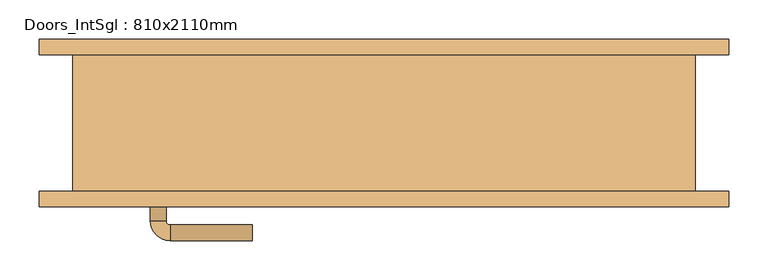
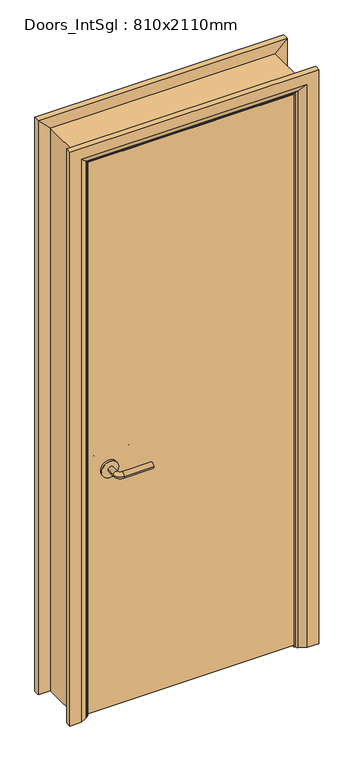
"""IFC4 building model written with IfcOpenShell, lengths in millimetres: door geometry, Doors_IntSgl : 810x2110mm."""

from ifc_helpers import new_model, si_unit, point, frame, frame_2d, origin, place, context, project, spatial, polyline, circle_curve, ellipse_curve, trimmed, segment, composite_curve, outline, extrude, faceted_brep, source, transform, mapped, element, save
from ifc_brep_helpers import plane_surface, cylinder_surface, revolved_surface, advanced_brep


def doors_intsgl_810x2110mm_f0bad3dc(model_context):
    return source(origin(), model_context, "Body", "SolidModel", [
        advanced_brep(
        [(-298.0, -40.868, 900.0), (-278.0, -40.868, 900.0), (-298.0, -10.868, 900.0), (-278.0, -10.868, 900.0), (-273.0, -5.868, 900.0), (-273.0, 14.132, 900.0), (-168.0, 14.132, 900.0), (-168.0, -5.868, 900.0)],
        [
            (0, 1, circle_curve(frame((-288.0, -40.868, 900.0), z_axis=(0.0, -1.0, 0.0), x_axis=(1.0, 0.0, 0.0)), 10.0)),
            (1, 0, circle_curve(frame((-288.0, -40.868, 900.0), z_axis=(0.0, -1.0, 0.0), x_axis=(1.0, 0.0, 0.0)), 10.0)),
            (0, 2),
            (2, 3, circle_curve(frame((-288.0, -10.868, 900.0), z_axis=(0.0, -1.0, 0.0), x_axis=(1.0, 0.0, 0.0)), 10.0)),
            (3, 1),
            (3, 2, circle_curve(frame((-288.0, -10.868, 900.0), z_axis=(0.0, -1.0, 0.0), x_axis=(1.0, 0.0, 0.0)), 10.0)),
            (4, 3, circle_curve(frame((-273.0, -10.868, 900.0), z_axis=(0.0, 0.0, 1.0), x_axis=(-1.0, 0.0, 0.0)), 5.0)),
            (2, 5, circle_curve(frame((-273.0, -10.868, 900.0), z_axis=(0.0, 0.0, -1.0), x_axis=(-1.0, 0.0, 0.0)), 25.0)),
            (5, 4, circle_curve(frame((-273.0, 4.132, 900.0), z_axis=(-1.0, 0.0, 0.0), x_axis=(0.0, -1.0, 0.0)), 10.0)),
            (4, 5, circle_curve(frame((-273.0, 4.132, 900.0), z_axis=(-1.0, 0.0, 0.0), x_axis=(0.0, -1.0, 0.0)), 10.0)),
            (6, 7, circle_curve(frame((-168.0, 4.132, 900.0), z_axis=(1.0, 0.0, 0.0), x_axis=(0.0, -1.0, 0.0)), 10.0)),
            (7, 6, circle_curve(frame((-168.0, 4.132, 900.0), z_axis=(1.0, 0.0, 0.0), x_axis=(0.0, -1.0, 0.0)), 10.0)),
            (5, 6),
            (7, 4),
        ],
        [
            plane_surface(frame((-288.0, -40.868, 900.0), z_axis=(0.0, -1.0, 0.0), x_axis=(0.0, 0.0, 1.0))),
            cylinder_surface(frame((-288.0, -40.868, 900.0), z_axis=(0.0, -1.0, 0.0), x_axis=(1.0, 0.0, 0.0)), 10.0),
            revolved_surface(trimmed(ellipse_curve(frame((-288.0, -10.868, 900.0), z_axis=(0.0, -1.0, 0.0), x_axis=(1.0, 0.0, 0.0)), 10.0, 10.0), [point((-298.0, -10.868, 900.0))], [point((-278.0, -10.868, 900.0))], True, "CARTESIAN"), (-273.0, -10.868, 900.0), (0.0, 0.0, -1.0)),
            revolved_surface(trimmed(ellipse_curve(frame((-288.0, -10.868, 900.0), z_axis=(0.0, -1.0, 0.0), x_axis=(1.0, 0.0, 0.0)), 10.0, 10.0), [point((-278.0, -10.868, 900.0))], [point((-298.0, -10.868, 900.0))], True, "CARTESIAN"), (-273.0, -10.868, 900.0), (0.0, 0.0, -1.0)),
            plane_surface(frame((-168.0, 4.132, 900.0), z_axis=(1.0, 0.0, 0.0), x_axis=(0.0, 0.0, 1.0))),
            cylinder_surface(frame((-273.0, 4.132, 900.0), z_axis=(-1.0, 0.0, 0.0), x_axis=(0.0, -1.0, 0.0)), 10.0),
        ],
        [
            (0, [[1, 2]]),
            (1, [[-1, 3, 4, 5]]),
            (1, [[-2, -5, 6, -3]]),
            (2, [[7, -4, 8, 9]]),
            (3, [[-8, -6, -7, 10]]),
            (4, [[11, 12]]),
            (5, [[-9, 13, -12, 14]]),
            (5, [[-10, -14, -11, -13]]),
        ],
    ),
        extrude(outline(composite_curve([segment(trimmed(circle_curve(frame_2d((900.0, -290.5)), 30.0), [point((900.0, -320.5))], [point((900.0, -260.5))], False, "CARTESIAN"), True, "CONTINUOUS"), segment(trimmed(circle_curve(frame_2d((900.0, -290.5)), 30.0), [point((900.0, -260.5))], [point((900.0, -320.5))], False, "CARTESIAN"), True, "CONTINUOUS")], self_intersect=False)), frame((0.0, -48.868, 0.0), z_axis=(0.0, 1.0, 0.0), x_axis=(0.0, 0.0, 1.0)), (0.0, 0.0, 1.0), 8.0),
        advanced_brep(
        [(-298.0, -94.868, 900.0), (-278.0, -94.868, 900.0), (-278.0, -124.868, 900.0), (-298.0, -124.868, 900.0), (-273.0, -129.868, 900.0), (-273.0, -149.868, 900.0), (-168.0, -149.868, 900.0), (-168.0, -129.868, 900.0)],
        [
            (0, 1, circle_curve(frame((-288.0, -94.868, 900.0), z_axis=(0.0, 1.0, 0.0), x_axis=(1.0, 0.0, 0.0)), 10.0)),
            (1, 0, circle_curve(frame((-288.0, -94.868, 900.0), z_axis=(0.0, 1.0, 0.0), x_axis=(1.0, 0.0, 0.0)), 10.0)),
            (1, 2),
            (2, 3, circle_curve(frame((-288.0, -124.868, 900.0), z_axis=(0.0, 1.0, 0.0), x_axis=(1.0, 0.0, 0.0)), 10.0)),
            (3, 0),
            (3, 2, circle_curve(frame((-288.0, -124.868, 900.0), z_axis=(0.0, 1.0, 0.0), x_axis=(1.0, 0.0, 0.0)), 10.0)),
            (4, 5, circle_curve(frame((-273.0, -139.868, 900.0), z_axis=(-1.0, 0.0, 0.0), x_axis=(0.0, 1.0, 0.0)), 10.0)),
            (5, 3, circle_curve(frame((-273.0, -124.868, 900.0), z_axis=(0.0, 0.0, -1.0), x_axis=(-1.0, 0.0, 0.0)), 25.0)),
            (2, 4, circle_curve(frame((-273.0, -124.868, 900.0), z_axis=(0.0, 0.0, 1.0), x_axis=(-1.0, 0.0, 0.0)), 5.0)),
            (5, 4, circle_curve(frame((-273.0, -139.868, 900.0), z_axis=(-1.0, 0.0, 0.0), x_axis=(0.0, 1.0, 0.0)), 10.0)),
            (6, 7, circle_curve(frame((-168.0, -139.868, 900.0), z_axis=(1.0, 0.0, 0.0), x_axis=(0.0, 1.0, 0.0)), 10.0)),
            (7, 6, circle_curve(frame((-168.0, -139.868, 900.0), z_axis=(1.0, 0.0, 0.0), x_axis=(0.0, 1.0, 0.0)), 10.0)),
            (4, 7),
            (6, 5),
        ],
        [
            plane_surface(frame((-288.0, -94.868, 900.0), z_axis=(0.0, 1.0, 0.0), x_axis=(0.0, 0.0, 1.0))),
            cylinder_surface(frame((-288.0, -94.868, 900.0), z_axis=(0.0, 1.0, 0.0), x_axis=(1.0, 0.0, 0.0)), 10.0),
            revolved_surface(trimmed(ellipse_curve(frame((-288.0, -124.868, 900.0), z_axis=(0.0, -1.0, 0.0), x_axis=(1.0, 0.0, 0.0)), 10.0, 10.0), [point((-298.0, -124.868, 900.0))], [point((-278.0, -124.868, 900.0))], True, "CARTESIAN"), (-273.0, -124.868, 900.0), (0.0, 0.0, -1.0)),
            revolved_surface(trimmed(ellipse_curve(frame((-288.0, -124.868, 900.0), z_axis=(0.0, -1.0, 0.0), x_axis=(1.0, 0.0, 0.0)), 10.0, 10.0), [point((-278.0, -124.868, 900.0))], [point((-298.0, -124.868, 900.0))], True, "CARTESIAN"), (-273.0, -124.868, 900.0), (0.0, 0.0, -1.0)),
            plane_surface(frame((-168.0, -139.868, 900.0), z_axis=(1.0, 0.0, 0.0), x_axis=(0.0, 0.0, 1.0))),
            cylinder_surface(frame((-273.0, -139.868, 900.0), z_axis=(-1.0, 0.0, 0.0), x_axis=(0.0, 1.0, 0.0)), 10.0),
        ],
        [
            (0, [[1, 2]]),
            (1, [[3, 4, 5, -2]]),
            (1, [[-5, 6, -3, -1]]),
            (2, [[7, 8, -4, 9]]),
            (3, [[10, -9, -6, -8]]),
            (4, [[11, 12]]),
            (5, [[13, -11, 14, -7]]),
            (5, [[-14, -12, -13, -10]]),
        ],
    ),
        extrude(outline(composite_curve([segment(trimmed(circle_curve(frame_2d((900.0, -290.5)), 30.0), [point((900.0, -320.5))], [point((900.0, -260.5))], False, "CARTESIAN"), True, "CONTINUOUS"), segment(trimmed(circle_curve(frame_2d((900.0, -290.5)), 30.0), [point((900.0, -260.5))], [point((900.0, -320.5))], False, "CARTESIAN"), True, "CONTINUOUS")], self_intersect=False)), frame((0.0, -94.868, 0.0), z_axis=(0.0, 1.0, 0.0), x_axis=(0.0, 0.0, 1.0)), (0.0, 0.0, 1.0), 8.0),
        extrude(outline(polyline([(363.0, -48.868), (363.0, -86.868), (-363.0, -86.868), (-363.0, -48.868), (363.0, -48.868)])), frame((0.0, 0.0, 8.0), z_axis=(0.0, 0.0, 1.0), x_axis=(1.0, 0.0, 0.0)), (0.0, 0.0, 1.0), 2060.0),
        advanced_brep(
        [(440.0, -106.868, 0.0), (400.0, -106.868, 0.0), (374.0, -92.868, 0.0), (370.0, -86.868, 0.0), (440.0, -86.868, 0.0), (440.0, -86.868, 2145.0), (440.0, -106.868, 2145.0), (370.0, -86.868, 2075.0), (-370.0, -86.868, 2075.0), (-370.0, -86.868, 0.0), (-440.0, -86.868, 0.0), (-440.0, -86.868, 2145.0), (374.0, -92.868, 2079.0), (400.0, -106.868, 2105.0), (-440.0, -106.868, 2145.0), (-440.0, -106.868, 0.0), (-400.0, -106.868, 0.0), (-400.0, -106.868, 2105.0), (-374.0, -92.868, 2079.0), (-374.0, -92.868, 0.0)],
        [
            (0, 1),
            (1, 2),
            (2, 3, circle_curve(frame((378.0, -85.868, 0.0), z_axis=(0.0, 0.0, -1.0), x_axis=(1.0, 0.0, 0.0)), 8.0622577)),
            (3, 4),
            (4, 0),
            (4, 5),
            (5, 6),
            (6, 0),
            (3, 7),
            (7, 8),
            (8, 9),
            (9, 10),
            (10, 11),
            (11, 5),
            (2, 12),
            (12, 7, ellipse_curve(frame((378.0, -85.868, 2083.0), z_axis=(0.7071067811865475, 0.0, -0.7071067811865475), x_axis=(-0.7071067811865474, 0.0, -0.7071067811865476)), 11.4017543, 8.0622577)),
            (1, 13),
            (13, 12),
            (6, 14),
            (14, 15),
            (15, 16),
            (16, 17),
            (17, 13),
            (11, 14),
            (12, 18),
            (18, 8, ellipse_curve(frame((-378.0, -85.868, 2083.0), z_axis=(0.7071067811865475, 0.0, 0.7071067811865475), x_axis=(0.7071067811865476, 0.0, -0.7071067811865474)), 11.4017543, 8.0622577)),
            (17, 18),
            (15, 10),
            (9, 19, circle_curve(frame((-378.0, -85.868, 0.0), z_axis=(0.0, 0.0, -1.0), x_axis=(-1.0, 0.0, 0.0)), 8.0622577)),
            (19, 16),
            (18, 19),
        ],
        [
            plane_surface(frame((370.0, -86.868, 0.0), z_axis=(0.0, 0.0, -1.0), x_axis=(0.0, 1.0, 0.0))),
            plane_surface(frame((440.0, -106.868, 0.0), z_axis=(1.0, 0.0, 0.0), x_axis=(0.0, 0.0, 1.0))),
            plane_surface(frame((440.0, -86.868, 0.0), z_axis=(0.0, 1.0, 0.0), x_axis=(0.0, 0.0, 1.0))),
            cylinder_surface(frame((378.0, -85.868, 0.0), z_axis=(0.0, 0.0, -1.0), x_axis=(1.0, 0.0, 0.0)), 8.0622577),
            plane_surface(frame((374.0, -92.868, 0.0), z_axis=(-0.4740998230350126, -0.880471099922178, 0.0), x_axis=(0.0, 0.0, 1.0))),
            plane_surface(frame((400.0, -106.868, 0.0), z_axis=(0.0, -1.0, 0.0), x_axis=(0.0, 0.0, 1.0))),
            plane_surface(frame((440.0, -106.868, 2145.0), z_axis=(0.0, 0.0, 1.0), x_axis=(-1.0, 0.0, 0.0))),
            cylinder_surface(frame((370.0, -85.868, 2083.0), z_axis=(1.0, 0.0, 0.0), x_axis=(0.0, 0.0, 1.0)), 8.0622577),
            plane_surface(frame((374.0, -92.868, 2079.0), z_axis=(0.0, -0.8804710999221764, -0.4740998230350154), x_axis=(-1.0, 0.0, 0.0))),
            plane_surface(frame((-370.0, -86.868, 0.0), z_axis=(0.0, 0.0, -1.0), x_axis=(0.0, 1.0, 0.0))),
            plane_surface(frame((-440.0, -106.868, 2145.0), z_axis=(-1.0, 0.0, 0.0), x_axis=(0.0, 0.0, -1.0))),
            cylinder_surface(frame((-378.0, -85.868, 2075.0), z_axis=(0.0, 0.0, 1.0), x_axis=(-1.0, 0.0, 0.0)), 8.0622577),
            plane_surface(frame((-374.0, -92.868, 2079.0), z_axis=(0.47409982303501824, -0.8804710999221749, 0.0), x_axis=(0.0, 0.0, -1.0))),
        ],
        [
            (0, [[1, 2, 3, 4, 5]]),
            (1, [[6, 7, 8, -5]]),
            (2, [[9, 10, 11, 12, 13, 14, -6, -4]]),
            (3, [[15, 16, -9, -3]]),
            (4, [[17, 18, -15, -2]]),
            (5, [[-8, 19, 20, 21, 22, 23, -17, -1]]),
            (6, [[-14, 24, -19, -7]]),
            (7, [[25, 26, -10, -16]]),
            (8, [[-23, 27, -25, -18]]),
            (9, [[28, -12, 29, 30, -21]]),
            (10, [[-13, -28, -20, -24]]),
            (11, [[31, -29, -11, -26]]),
            (12, [[-22, -30, -31, -27]]),
        ],
    ),
        extrude(outline(polyline([(0.0, -346.0), (2051.0, -346.0), (2051.0, 346.0), (0.0, 346.0), (0.0, 365.0), (2070.0, 365.0), (2070.0, -365.0), (0.0, -365.0), (0.0, -346.0)])), frame((0.0, -46.868, 0.0), z_axis=(0.0, 1.0, 0.0), x_axis=(0.0, 0.0, 1.0)), (0.0, 0.0, 1.0), 32.0),
        advanced_brep(
        [(-440.0, 106.868, 0.0), (-400.0, 106.868, 0.0), (-374.0, 92.868, 0.0), (-370.0, 86.868, 0.0), (-440.0, 86.868, 0.0), (-440.0, 86.868, 2145.0), (-440.0, 106.868, 2145.0), (-370.0, 86.868, 2075.0), (-374.0, 92.868, 2079.0), (-400.0, 106.868, 2105.0), (440.0, 86.868, 2145.0), (440.0, 106.868, 2145.0), (370.0, 86.868, 2075.0), (374.0, 92.868, 2079.0), (400.0, 106.868, 2105.0), (440.0, 106.868, 0.0), (440.0, 86.868, 0.0), (370.0, 86.868, 0.0), (374.0, 92.868, 0.0), (400.0, 106.868, 0.0)],
        [
            (0, 1),
            (1, 2),
            (2, 3, circle_curve(frame((-378.0, 85.868, 0.0), z_axis=(0.0, 0.0, -1.0), x_axis=(-1.0, 0.0, 0.0)), 8.0622577)),
            (3, 4),
            (4, 0),
            (4, 5),
            (5, 6),
            (6, 0),
            (3, 7),
            (7, 5),
            (2, 8),
            (8, 7, ellipse_curve(frame((-378.0, 85.868, 2083.0), z_axis=(-0.7071067811865475, 0.0, -0.7071067811865475), x_axis=(0.7071067811865474, 0.0, -0.7071067811865476)), 11.4017543, 8.0622577)),
            (1, 9),
            (9, 8),
            (6, 9),
            (5, 10),
            (10, 11),
            (11, 6),
            (7, 12),
            (12, 10),
            (8, 13),
            (13, 12, ellipse_curve(frame((378.0, 85.868, 2083.0), z_axis=(-0.7071067811865475, 0.0, 0.7071067811865475), x_axis=(-0.7071067811865476, 0.0, -0.7071067811865474)), 11.4017543, 8.0622577)),
            (9, 14),
            (14, 13),
            (11, 14),
            (15, 16),
            (16, 17),
            (17, 18, circle_curve(frame((378.0, 85.868, 0.0), z_axis=(0.0, 0.0, -1.0), x_axis=(1.0, 0.0, 0.0)), 8.0622577)),
            (18, 19),
            (19, 15),
            (10, 16),
            (15, 11),
            (12, 17),
            (13, 18),
            (14, 19),
        ],
        [
            plane_surface(frame((-370.0, 159.6690989, 0.0), z_axis=(0.0, 0.0, -1.0), x_axis=(1.0, 0.0, 0.0))),
            plane_surface(frame((-440.0, 106.868, 0.0), z_axis=(-1.0, 0.0, 0.0), x_axis=(0.0, 0.0, 1.0))),
            plane_surface(frame((-440.0, 86.868, 0.0), z_axis=(0.0, -1.0, 0.0), x_axis=(0.0, 0.0, 1.0))),
            cylinder_surface(frame((-378.0, 85.868, 0.0), z_axis=(0.0, 0.0, -1.0), x_axis=(-1.0, 0.0, 0.0)), 8.0622577),
            plane_surface(frame((-374.0, 92.868, 0.0), z_axis=(0.4740998230350183, 0.8804710999221749, 0.0), x_axis=(0.0, 0.0, 1.0))),
            plane_surface(frame((-400.0, 106.868, 0.0), z_axis=(0.0, 1.0, 0.0), x_axis=(0.0, 0.0, 1.0))),
            plane_surface(frame((-440.0, 106.868, 2145.0), z_axis=(0.0, 0.0, 1.0), x_axis=(1.0, 0.0, 0.0))),
            plane_surface(frame((-440.0, 86.868, 2145.0), z_axis=(0.0, -1.0, 0.0), x_axis=(1.0, 0.0, 0.0))),
            cylinder_surface(frame((-370.0, 85.868, 2083.0), z_axis=(-1.0, 0.0, 0.0), x_axis=(0.0, 0.0, 1.0)), 8.0622577),
            plane_surface(frame((-374.0, 92.868, 2079.0), z_axis=(0.0, 0.8804710999221749, -0.4740998230350183), x_axis=(1.0, 0.0, 0.0))),
            plane_surface(frame((-400.0, 106.868, 2105.0), z_axis=(0.0, 1.0, 0.0), x_axis=(1.0, 0.0, 0.0))),
            plane_surface(frame((370.0, 159.6690989, 0.0), z_axis=(0.0, 0.0, -1.0), x_axis=(-1.0, 0.0, 0.0))),
            plane_surface(frame((440.0, 106.868, 2145.0), z_axis=(1.0, 0.0, 0.0), x_axis=(0.0, 0.0, -1.0))),
            plane_surface(frame((440.0, 86.868, 2145.0), z_axis=(0.0, -1.0, 0.0), x_axis=(0.0, 0.0, -1.0))),
            cylinder_surface(frame((378.0, 85.868, 2075.0), z_axis=(0.0, 0.0, 1.0), x_axis=(1.0, 0.0, 0.0)), 8.0622577),
            plane_surface(frame((374.0, 92.868, 2079.0), z_axis=(-0.4740998230350183, 0.8804710999221749, 0.0), x_axis=(0.0, 0.0, -1.0))),
            plane_surface(frame((400.0, 106.868, 2105.0), z_axis=(0.0, 1.0, 0.0), x_axis=(0.0, 0.0, -1.0))),
        ],
        [
            (0, [[1, 2, 3, 4, 5]]),
            (1, [[6, 7, 8, -5]]),
            (2, [[9, 10, -6, -4]]),
            (3, [[11, 12, -9, -3]]),
            (4, [[13, 14, -11, -2]]),
            (5, [[-8, 15, -13, -1]]),
            (6, [[16, 17, 18, -7]]),
            (7, [[19, 20, -16, -10]]),
            (8, [[21, 22, -19, -12]]),
            (9, [[23, 24, -21, -14]]),
            (10, [[-18, 25, -23, -15]]),
            (11, [[26, 27, 28, 29, 30]]),
            (12, [[31, -26, 32, -17]]),
            (13, [[33, -27, -31, -20]]),
            (14, [[34, -28, -33, -22]]),
            (15, [[35, -29, -34, -24]]),
            (16, [[-32, -30, -35, -25]]),
        ],
    ),
        faceted_brep([(-365.0, -86.868, 0.0), (-397.0, -86.868, 0.0), (-397.0, 86.868, 0.0), (-365.0, 86.868, 0.0), (-365.0, 86.868, 2070.0), (-365.0, -86.868, 2070.0), (-397.0, 86.868, 2102.0), (-397.0, -86.868, 2102.0), (365.0, 86.868, 2070.0), (365.0, -86.868, 2070.0), (397.0, 86.868, 2102.0), (397.0, -86.868, 2102.0), (365.0, -86.868, 0.0), (365.0, 86.868, 0.0), (397.0, 86.868, 0.0), (397.0, -86.868, 0.0)], [[[0, 1, 2, 3]], [[3, 4, 5, 0]], [[2, 6, 4, 3]], [[1, 7, 6, 2]], [[0, 5, 7, 1]], [[4, 8, 9, 5]], [[6, 10, 8, 4]], [[7, 11, 10, 6]], [[5, 9, 11, 7]], [[12, 13, 14, 15]], [[8, 13, 12, 9]], [[10, 14, 13, 8]], [[11, 15, 14, 10]], [[9, 12, 15, 11]]]),
    ])


if __name__ == "__main__":
    model = new_model("IFC4")
    model_context = context("Model", 3, world=origin())
    ifc_project = project(units=[si_unit("LENGTHUNIT", "METRE", prefix="MILLI")], contexts=[model_context])
    site = spatial("IfcSite", under=ifc_project)
    building = spatial("IfcBuilding", under=site)
    placement = place(None, origin())
    doors_intsgl_810x2110mm_shape = doors_intsgl_810x2110mm_f0bad3dc(model_context)
    element("IfcDoor", 1, ObjectType="Doors_IntSgl : 810x2110mm", at=placement, inside=building, context=model_context, shape_type="MappedRepresentation", body=[
        mapped(doors_intsgl_810x2110mm_shape, transform((0.0, 0.0, 0.0), x_axis=(1.0, 0.0, 0.0), y_axis=(0.0, 1.0, 0.0), z_axis=(0.0, 0.0, 1.0))),
    ])
    save(model, "model.ifc")

# Revit data of these elements
# Type "Doors_IntSgl : 810x2110mm"
#   Construction Type Id = "MDOOR"
#   Type Mark = "42"
#   Type Comments = "Internal Single"
#   Operation = "SingleSwingRight"
#   Manufacturer = "Revit"
#   Keynote = "L20"
#   Description = "Internal Single Door"
#   Analytic Construction = "Metal"
#   UnderCut = 0.026247 ft
#   Tolerance = 0.006562 ft
#   Thickness = 0.124672 ft
#   Thermal Resistance (R) = 0.270117 (m²·K)/W
#   Structural Tolerance = 0.026247 ft
#   StopDepth = 0.104987 ft
#   Stop Thickness = 0.062336 ft
#   Rough Width = 2.65748 ft
#   Rough Height = 6.922572 ft
#   Height to Top Lock Rail = 3.28084 ft
#   Heat Transfer Coefficient (U) = 3.7021 W/(m²·K)
#   Handle Z Distance = 2.952756 ft
#   Handle X Distance = 0.246063 ft
#   Frame Thickness = 0.104987 ft
#   Door Panel Width = 2.38189 ft
#   Door Panel Thickness = 0.124672 ft
#   Door Panel Offset = 0.0 ft
#   Height = 6.922572 ft
#   Width = 2.65748 ft
#   Door Panel Height = 6.75853 ft
#   Architrave Setback = 0.016404 ft
#   Define Thermal Properties by = 1
#   Vis - Ironmongery = yes
#   Material Ironmongery = Door - Handle
#   Material Frame = Door - Frame/Mullion (1)
#   Material Door = Door - Panel
#   Material Architrave = Door - Architrave
#   Visual Light Transmittance = 0
#   Solar Heat Gain Coefficient = 0
#   Function = (empty or 0)
#   Wall Closure = (empty or 0)
# Element 1 (IfcDoor, "Doors_IntSgl : 810x2110mm")
#   Materials on its faces: "Door - Architrave", "Door - Handle", "Door - Frame/Mullion (1)", "Door - Panel"
# Materials
#   "Door - Handle": colour RGB 0 0 0, transparency 0, Keynote = "P21", Cost = 0
#   "Door - Frame/Mullion (1)": class "Wood", colour RGB 212 179 113, transparency 0, Keynote = "L20", Cost = 0
#   "Door - Panel": class "Wood", colour RGB 210 159 95, transparency 0, Keynote = "L20", Cost = 0
#   "Door - Architrave": class "Wood", colour RGB 154 90 5, transparency 0, Keynote = "P20", Cost = 0
